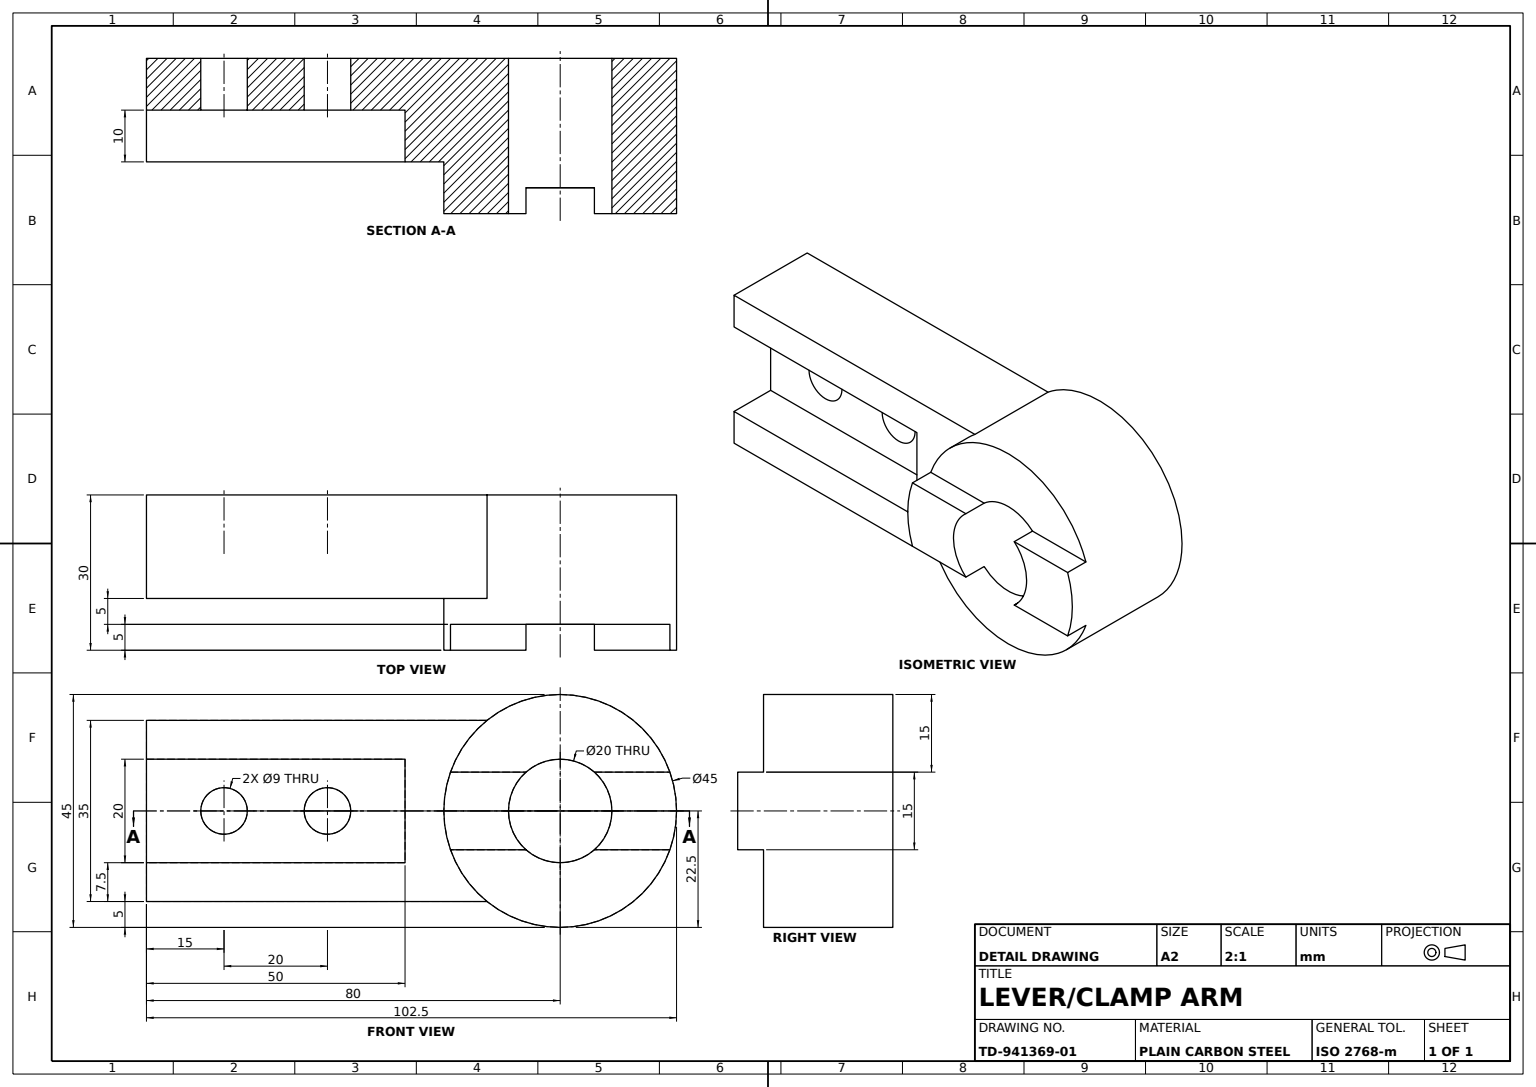
SolidWorks part; units mm, degrees
material "Plain Carbon Steel"
ref_plane "Front Plane" through (0, 0, 0) normal (0, 0, 1) x (1, 0, 0)
ref_plane "Top Plane" through (0, 0, 0) normal (0, 1, 0) x (1, 0, 0)
ref_plane "Right Plane" through (0, 0, 0) normal (1, 0, 0) x (0, 0, -1)
sketch "Hub Profile Sketch" plane through (0, 0, 0) normal (1, 0, 0) x (0, 0, -1)
  circle A0 centre (0, 0) radius 22.5
  circle A1 centre (0, 0) radius 10
  dimension "D1" = 45
  dimension "D2" = 20
extrude "Hub Boss Ø45" add sketch "Hub Profile Sketch" along normal blind 30
sketch "Hub Face Slot Sketch" plane through (30, 0, 0) normal (1, 0, 0) x (0, 0, -1)
  line L0 (-21.2132, 7.5) -> (21.2132, 7.5)
  line L1 (-21.2132, -7.5) -> (21.2132, -7.5)
  circle A0 centre (0, 0) radius 22.5 construction
  arc A1 (-21.2132, 7.5) -> (21.2132, 7.5) centre (0, 0) cw
  arc A2 (-21.2132, -7.5) -> (21.2132, -7.5) centre (0, 0) ccw
  dimension "D1" = 15
extrude "Hub Face Slot 15" cut sketch "Hub Face Slot Sketch" against normal blind 5 contours L0 A1
sketch "Hub Slot Step Sketch" plane through (30, 0, 0) normal (1, 0, 0) x (0, 0, -1)
  line L0 (-21.2132, -7.5) -> (21.2132, -7.5)
  line L1 (6.6144, 7.5) -> (21.2132, 7.5) construction
  arc A0 (-21.2132, 7.5) -> (21.2132, 7.5) centre (0, 0) ccw construction
  arc A1 (-21.2132, -7.5) -> (21.2132, -7.5) centre (0, 0) ccw
  dimension "D1" = 15
extrude "Hub Slot Step 15" cut sketch "Hub Slot Step Sketch" against normal blind 5
sketch "Crank Arm Profile Sketch" plane through (0, 0, 0) normal (0, 0, 1) x (1, 0, 0)
  line L0 (-10.416, 0) -> (40.918, 0) construction
  line L1 (0, 22.5) -> (0, -22.5) construction
  line L2 (20, -17.5) -> (0, -17.5)
  line L3 (20, -17.5) -> (20, 17.5)
  line L4 (20, 17.5) -> (0, 17.5)
  line L5 (0, -17.5) -> (0, 17.5)
  line L6 (20, -17.5) -> (0, 17.5) construction
  line L7 (20, 17.5) -> (0, -17.5) construction
  point P3 (10, 0)
  point P8 (0, 0)
  dimension "D1" = 20
  dimension "D2" = 35
extrude "Crank Arm" add sketch "Crank Arm Profile Sketch" along normal blind 80
sketch "Bore Sketch" plane through (20, 0, 0) normal (1, 0, 0) x (0, 0, -1)
  circle A0 centre (0, 0) radius 10
  dimension "D1" = 20
extrude "Bore Ø20" cut sketch "Bore Sketch" against normal blind 80
sketch "Arm Window Sketch" plane through (0, 0, 80) normal (0, 0, 1) x (1, 0, 0)
  line L0 (20, -17.5) -> (20, 17.5) construction
  line L1 (0, 17.5) -> (0, -17.5) construction
  line L2 (20, -10) -> (10, -10)
  line L3 (20, -10) -> (20, 10)
  line L4 (20, 10) -> (10, 10)
  line L5 (10, -10) -> (10, 10)
  point P8 (0, 0)
  point P9 (10, 0)
  dimension "D1" = 10
  dimension "D2" = 20
extrude "Arm Window 10x20" cut sketch "Arm Window Sketch" against normal blind 50 contours L5 L4 L3 L2
sketch "Arm Side Cut Sketch" plane through (10, 0, 0) normal (1, 0, 0) x (0, 0, -1)
  line L0 (-80, 0) -> (-26.4304, 0) construction
  line L1 (-80, -10) -> (-80, 10) construction
  circle A0 centre (-65, 0) radius 4.5
  circle A1 centre (-45, 0) radius 4.5
  dimension "D3" = 9
  dimension "D1" = 15
  dimension "D2" = 20
extrude "Arm Side Cut" cut sketch "Arm Side Cut Sketch" against normal through all
